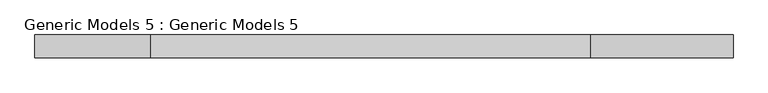
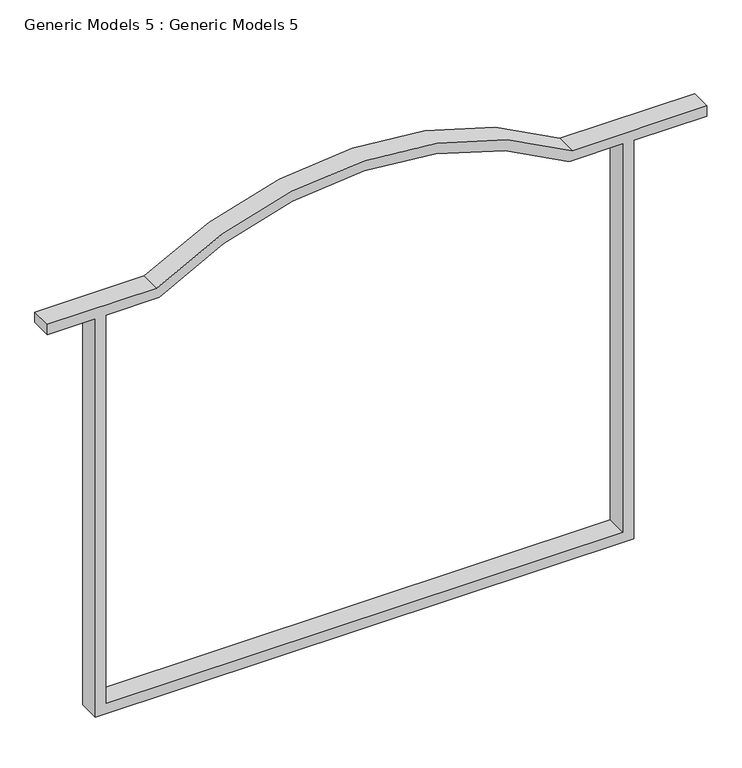
"""IFC4 building model written with IfcOpenShell, lengths in millimetres: proxy geometry, Generic Models 5 : Generic Models 5."""

from ifc_helpers import new_model, si_unit, point, frame, frame_2d, origin, place, context, project, spatial, polyline, circle_curve, trimmed, segment, composite_curve, outline, extrude, source, transform, mapped, element, save


def generic_models_5_generic_models_5_33064adf(model_context):
    return source(origin(), model_context, "Body", "SweptSolid", [
        extrude(outline(composite_curve([segment(trimmed(circle_curve(frame_2d((4226.2703785, -9842.3236584)), 1788.8851029), [point((5722.5214447, -8861.8428283))], [point((5722.5214447, -10822.8044885))], False, "CARTESIAN"), True, "CONTINUOUS"), segment(polyline([(5722.5214447, -10822.8044885), (5722.5214447, -11339.0293601), (5671.7214447, -11339.0293601), (5671.7214447, -11112.3236584), (3683.3026126, -11112.3236584), (3683.3026126, -8572.3236584), (5671.7214447, -8572.3236584), (5671.7214447, -8226.1270642), (5722.5214447, -8226.1270642), (5722.5214447, -8861.8428283)]), True, "CONTINUOUS")], self_intersect=False), holes=[composite_curve([segment(polyline([(5671.7214447, -11061.5236584), (5671.7214447, -10807.5236584)]), True, "CONTINUOUS"), segment(trimmed(circle_curve(frame_2d((4226.2703785, -9842.3236584)), 1738.0851029), [point((5671.7214447, -10807.5236584))], [point((5671.7214447, -8877.1236584))], True, "CARTESIAN"), True, "CONTINUOUS"), segment(polyline([(5671.7214447, -8877.1236584), (5671.7214447, -8623.1236584), (3734.1026126, -8623.1236584), (3734.1026126, -11061.5236584), (5671.7214447, -11061.5236584)]), True, "CONTINUOUS")], self_intersect=False)]), frame((0.0, -13589.402305, 0.0), z_axis=(0.0, 1.0, 0.0), x_axis=(0.0, 0.0, 1.0)), (0.0, 0.0, 1.0), 101.6),
    ])


if __name__ == "__main__":
    model = new_model("IFC4")
    model_context = context("Model", 3, world=origin())
    ifc_project = project(units=[si_unit("LENGTHUNIT", "METRE", prefix="MILLI")], contexts=[model_context])
    site = spatial("IfcSite", under=ifc_project)
    building = spatial("IfcBuilding", under=site)
    placement = place(None, origin())
    generic_models_5_generic_models_5_shape = generic_models_5_generic_models_5_33064adf(model_context)
    element("IfcBuildingElementProxy", 1, Name="Generic Models 5 : Generic Models 5", ObjectType="Generic Models 5 : Generic Models 5", at=placement, inside=building, context=model_context, shape_type="MappedRepresentation", body=[
        mapped(generic_models_5_generic_models_5_shape, transform((0.0, 0.0, 0.0), x_axis=(1.0, 0.0, 0.0), y_axis=(0.0, 1.0, 0.0), z_axis=(0.0, 0.0, 1.0))),
    ])
    save(model, "model.ifc")

# Revit data of these elements
# Element 1 (IfcBuildingElementProxy, "Generic Models 5 : Generic Models 5")
#   Materials on its faces: "ACCENT BEIGE COLOUR"
# Materials
#   "ACCENT BEIGE COLOUR": class "Generic", colour RGB 120 120 120, transparency 0, Cost = 0
